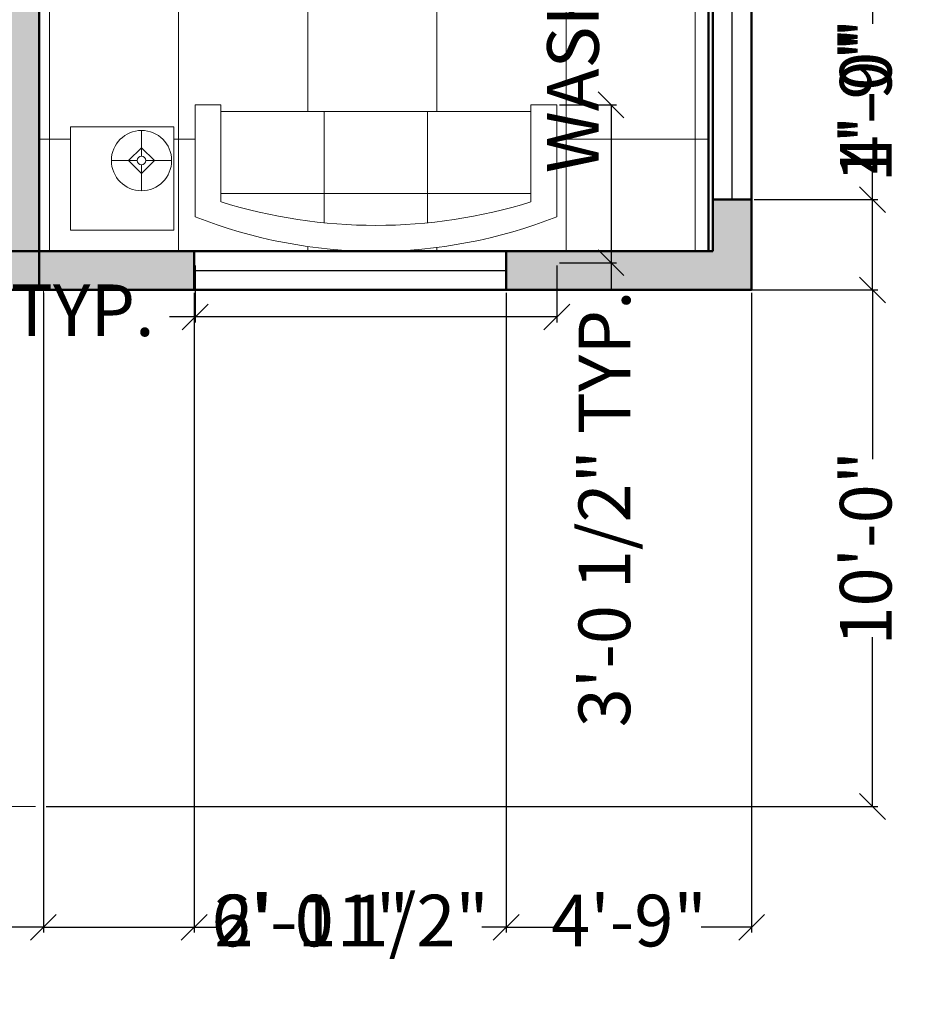
# Model space of a CAD drawing. Units: inches. Extents: x 2371 to 3019, y 129 to 700.
# Tile 10 of 14: x 2753 to 2959, y 129 to 358. Entities that reach past the tile are written whole.
import ezdxf

# ---------------------------------------------------------------- set-up
doc = ezdxf.new("R2010")
doc.units = ezdxf.units.IN
doc.linetypes.add('DASHED', pattern=[19.05, 12.7, -6.35])
for name, color, linetype, lineweight in [('A-ANNO-DIMS', 2, 'Continuous', 18), ('A-FLOR-OVHD', 20, 'DASHED', 18), ('A-FLOR-PATT', 252, 'Continuous', 13), ('A-FURN', 8, 'Continuous', 18), ('A-GLAZ', 4, 'Continuous', 25), ('A-WALL', 7, 'Continuous', 50), ('A-WALL-PATT', 8, 'Continuous', 13)]:
    doc.layers.add(name, color=color, linetype=linetype, lineweight=lineweight)
doc.styles.get("Standard").update_dxf_attribs({"font": 'arial.ttf'})
doc.dimstyles.new('ISO-25', dxfattribs={"dimtxt": 12, "dimasz": 6, "dimexe": 1.25, "dimexo": 0.625, "dimtad": 0, "dimdec": 1, "dimlunit": 3, "dimtxsty": 'Standard', "dimblk": 'OBLIQUE', "dimblk1": 'ORIGIN2', "dimblk2": 'OBLIQUE', "dimcen": 2.5, "dimadec": 0, "dimazin": 0, "dimtfac": 1, "dimtdec": 1, "dimtmove": 0, "dimatfit": 3, "dimldrblk": 'OBLIQUE', "dimfxl": 1, "dimarcsym": 0})

# ---------------------------------------------------------------- blocks, each defined once
blk = doc.blocks.new('Lamp - Table')
for p, q in [((0, 7), (0, 1)), ((0, 3), (-3, 0)), ((3, 0), (0, 3)), ((-1, 0), (-7, 0)), ((-3, 0), (0, -3)), ((0, -3), (3, 0)), ((1, 0), (7, 0)), ((0, -1), (0, -7))]:
    blk.add_line(p, q)
for radius in [7, 1]:
    blk.add_circle((0, 0), radius)
blk = doc.blocks.new('Sofa - Roundback 7 ft.')
for p, q in [((-12.00002, -32.4421), (-12.00003, -6.5971)), ((11.99997, -32.4421), (11.99998, -6.5971)), ((-36.000027, -34), (-36.000027, -11.4696)), ((-35.999844, -13.3819), (35.9998, -13.3819)), ((35.99998, -34), (35.99998, -11.4696)), ((-36.000027, -32.4421), (35.99998, -32.4421))]:
    blk.add_line(p, q)
for points in [[(-36.000027, -34), (-42.000027, -34), (-42.000027, -8)], [(41.99998, -8), (41.99998, -34), (35.99998, -34)]]:
    blk.add_lwpolyline(points)
for centre, radius, start, end in [((0, -114.25), 114.25, 68.43141, 111.5686), ((-0.00001, -127.1968), 121.1968, 72.72033, 107.2797)]:
    blk.add_arc(centre, radius, start, end)
blk = doc.blocks.new('_Oblique')
at = {"color": 0, "linetype": 'ByBlock', "lineweight": -2}
blk.add_line((-0.5, -0.5), (0.5, 0.5), dxfattribs=at)
blk = doc.blocks.new('*D20')
at = {"layer": 'A-ANNO-DIMS', "color": 0, "lineweight": -2, "transparency": 16777216}
for p, q in [((2793.86, 300.68), (2793.86, 287.46)), ((2877.86, 300.68), (2877.86, 287.46)), ((2793.86, 288.71), (2787.86, 288.71)), ((2877.86, 288.71), (2793.86, 288.71))]:
    blk.add_line(p, q, dxfattribs=at)
at = {"layer": 'Defpoints', "color": 0, "lineweight": 25, "transparency": 16777216}
for p in [(2793.86, 301.31), (2877.86, 301.31), (2793.86, 288.71)]:
    blk.add_point(p, dxfattribs=at)
at = {"layer": 'A-ANNO-DIMS', "color": 0, "lineweight": -2, "transparency": 16777216, "xscale": 6, "yscale": 6, "zscale": 6}
for p, rotation in [((2793.86, 288.71), 180.0000057391524), ((2877.86, 288.71), 5.7391524333e-06)]:
    blk.add_blockref('_Oblique', p, dxfattribs=dict(at, rotation=rotation))
at = {"layer": 'A-ANNO-DIMS', "color": 0, "transparency": 16777216, "insert": (2725.54, 288.71), "char_height": 12, "attachment_point": 5, "rotation": 0}
blk.add_mtext('SOFA 7\'-0" TYP.', dxfattribs=at)
blk = doc.blocks.new('_Origin2')
at = {"color": 0, "linetype": 'ByBlock', "lineweight": -2}
blk.add_line((-0.5, 0), (-1, 0), dxfattribs=at)
for radius in [0.5, 0.25]:
    blk.add_circle((0, 0), radius, dxfattribs=at)
blk = doc.blocks.new('*D21')
at = {"layer": 'A-ANNO-DIMS', "color": 0, "lineweight": -2, "transparency": 16777216}
for p, q in [((2878.48, 337.98), (2891.71, 337.98)), ((2890.46, 337.98), (2890.46, 301.31)), ((2878.48, 301.31), (2891.71, 301.31)), ((2890.46, 301.31), (2890.46, 295.31))]:
    blk.add_line(p, q, dxfattribs=at)
at = {"layer": 'Defpoints', "color": 0, "lineweight": 25, "transparency": 16777216}
for p in [(2877.86, 337.98), (2877.86, 301.31), (2890.46, 301.31)]:
    blk.add_point(p, dxfattribs=at)
at = {"layer": 'A-ANNO-DIMS', "color": 0, "lineweight": -2, "transparency": 16777216, "xscale": 6, "yscale": 6, "zscale": 6}
for p, rotation in [((2890.46, 337.98), 90), ((2890.46, 301.31), 270)]:
    blk.add_blockref('_Oblique', p, dxfattribs=dict(at, rotation=rotation))
at = {"layer": 'A-ANNO-DIMS', "color": 0, "transparency": 16777216, "insert": (2890.46, 244.13), "char_height": 12, "attachment_point": 5, "rotation": 90}
blk.add_mtext('3\'-0 1/2" TYP.', dxfattribs=at)
blk = doc.blocks.new('*D26')
at = {"layer": 'A-ANNO-DIMS', "color": 0, "lineweight": -2, "transparency": 16777216}
for p, q in [((2886.23, 560.02), (2881.92, 560.02)), ((2883.17, 560.02), (2883.17, 535.47)), ((2886.23, 535.47), (2881.92, 535.47)), ((2883.17, 535.47), (2883.17, 529.47))]:
    blk.add_line(p, q, dxfattribs=at)
at = {"layer": 'Defpoints', "color": 0, "lineweight": 25, "transparency": 16777216}
for p in [(2886.85, 560.02), (2883.17, 535.47), (2886.85, 535.47)]:
    blk.add_point(p, dxfattribs=at)
at = {"layer": 'A-ANNO-DIMS', "color": 0, "lineweight": -2, "transparency": 16777216, "xscale": 6, "yscale": 6, "zscale": 6}
for p, rotation in [((2883.17, 560.02), 90), ((2883.17, 535.47), 270)]:
    blk.add_blockref('_Oblique', p, dxfattribs=dict(at, rotation=rotation))
at = {"layer": 'A-ANNO-DIMS', "color": 0, "transparency": 16777216, "insert": (2883.17, 423.09), "char_height": 12, "attachment_point": 5, "rotation": 90}
blk.add_mtext('WASH BASIN 2\'-0 1/2" TYP.', dxfattribs=at)
blk = doc.blocks.new('*D53')
at = {"layer": 'A-ANNO-DIMS', "color": 0, "lineweight": -2, "transparency": 16777216}
for p, q in [((2572.61, 174.35), (2572.61, 145.68)), ((2758.61, 174.35), (2758.61, 145.68)), ((2572.61, 146.93), (2644.93, 146.93)), ((2758.61, 146.93), (2686.28, 146.93))]:
    blk.add_line(p, q, dxfattribs=at)
at = {"layer": 'Defpoints', "color": 0, "lineweight": 25, "transparency": 16777216}
for p in [(2572.61, 174.98), (2758.61, 174.98), (2758.61, 146.93)]:
    blk.add_point(p, dxfattribs=at)
at = {"layer": 'A-ANNO-DIMS', "color": 0, "lineweight": -2, "transparency": 16777216, "xscale": 6, "yscale": 6, "zscale": 6, "rotation": 180}
blk.add_blockref('_Oblique', (2572.61, 146.93), dxfattribs=at)
at = {"layer": 'A-ANNO-DIMS', "color": 0, "lineweight": -2, "transparency": 16777216, "xscale": 6, "yscale": 6, "zscale": 6}
blk.add_blockref('_Oblique', (2758.61, 146.93), dxfattribs=at)
at = {"layer": 'A-ANNO-DIMS', "color": 0, "transparency": 16777216, "insert": (2665.61, 146.93), "char_height": 12, "attachment_point": 5}
blk.add_mtext('15\'-6"', dxfattribs=at)
blk = doc.blocks.new('*D54')
at = {"layer": 'A-ANNO-DIMS', "color": 0, "lineweight": -2, "transparency": 16777216}
for p, q in [((2758.61, 294.35), (2758.61, 145.68)), ((2793.61, 294.35), (2793.61, 145.68)), ((2758.61, 146.93), (2793.61, 146.93)), ((2793.61, 146.93), (2799.61, 146.93))]:
    blk.add_line(p, q, dxfattribs=at)
at = {"layer": 'Defpoints', "color": 0, "lineweight": 25, "transparency": 16777216}
for p in [(2758.61, 294.98), (2793.61, 294.98), (2793.61, 146.93)]:
    blk.add_point(p, dxfattribs=at)
at = {"layer": 'A-ANNO-DIMS', "color": 0, "lineweight": -2, "transparency": 16777216, "xscale": 6, "yscale": 6, "zscale": 6, "rotation": 180}
blk.add_blockref('_Oblique', (2758.61, 146.93), dxfattribs=at)
at = {"layer": 'A-ANNO-DIMS', "color": 0, "lineweight": -2, "transparency": 16777216, "xscale": 6, "yscale": 6, "zscale": 6}
blk.add_blockref('_Oblique', (2793.61, 146.93), dxfattribs=at)
at = {"layer": 'A-ANNO-DIMS', "color": 0, "transparency": 16777216, "insert": (2820.94, 146.93), "char_height": 12, "attachment_point": 5}
blk.add_mtext('2\'-11"', dxfattribs=at)
blk = doc.blocks.new('*D55')
at = {"layer": 'A-ANNO-DIMS', "color": 0, "lineweight": -2, "transparency": 16777216}
for p, q in [((2793.61, 294.35), (2793.61, 145.68)), ((2866.11, 294.35), (2866.11, 145.68)), ((2793.61, 146.93), (2799.27, 146.93)), ((2866.11, 146.93), (2860.44, 146.93))]:
    blk.add_line(p, q, dxfattribs=at)
at = {"layer": 'Defpoints', "color": 0, "lineweight": 25, "transparency": 16777216}
for p in [(2793.61, 294.98), (2866.11, 294.98), (2866.11, 146.93)]:
    blk.add_point(p, dxfattribs=at)
at = {"layer": 'A-ANNO-DIMS', "color": 0, "lineweight": -2, "transparency": 16777216, "xscale": 6, "yscale": 6, "zscale": 6, "rotation": 180}
blk.add_blockref('_Oblique', (2793.61, 146.93), dxfattribs=at)
at = {"layer": 'A-ANNO-DIMS', "color": 0, "lineweight": -2, "transparency": 16777216, "xscale": 6, "yscale": 6, "zscale": 6}
blk.add_blockref('_Oblique', (2866.11, 146.93), dxfattribs=at)
at = {"layer": 'A-ANNO-DIMS', "color": 0, "transparency": 16777216, "insert": (2829.86, 146.93), "char_height": 12, "attachment_point": 5}
blk.add_mtext('6\'-0 1/2"', dxfattribs=at)
blk = doc.blocks.new('*D56')
at = {"layer": 'A-ANNO-DIMS', "color": 0, "lineweight": -2, "transparency": 16777216}
for p, q in [((2866.11, 294.35), (2866.11, 145.68)), ((2923.11, 294.35), (2923.11, 145.68)), ((2866.11, 146.93), (2877.79, 146.93)), ((2923.11, 146.93), (2911.42, 146.93))]:
    blk.add_line(p, q, dxfattribs=at)
at = {"layer": 'Defpoints', "color": 0, "lineweight": 25, "transparency": 16777216}
for p in [(2866.11, 294.98), (2923.11, 294.98), (2923.11, 146.93)]:
    blk.add_point(p, dxfattribs=at)
at = {"layer": 'A-ANNO-DIMS', "color": 0, "lineweight": -2, "transparency": 16777216, "xscale": 6, "yscale": 6, "zscale": 6, "rotation": 180}
blk.add_blockref('_Oblique', (2866.11, 146.93), dxfattribs=at)
at = {"layer": 'A-ANNO-DIMS', "color": 0, "lineweight": -2, "transparency": 16777216, "xscale": 6, "yscale": 6, "zscale": 6}
blk.add_blockref('_Oblique', (2923.11, 146.93), dxfattribs=at)
at = {"layer": 'A-ANNO-DIMS', "color": 0, "transparency": 16777216, "insert": (2894.61, 146.93), "char_height": 12, "attachment_point": 5}
blk.add_mtext('4\'-9"', dxfattribs=at)
blk = doc.blocks.new('*D57')
at = {"layer": 'A-ANNO-DIMS', "color": 0, "lineweight": -2, "transparency": 16777216}
for p, q in [((2759.23, 294.98), (2952.41, 294.98)), ((2951.16, 294.98), (2951.16, 255.65)), ((2951.16, 174.98), (2951.16, 214.3)), ((2759.23, 174.98), (2952.41, 174.98))]:
    blk.add_line(p, q, dxfattribs=at)
at = {"layer": 'Defpoints', "color": 0, "lineweight": 25, "transparency": 16777216}
for p in [(2758.61, 294.98), (2758.61, 174.98), (2951.16, 174.98)]:
    blk.add_point(p, dxfattribs=at)
at = {"layer": 'A-ANNO-DIMS', "color": 0, "lineweight": -2, "transparency": 16777216, "xscale": 6, "yscale": 6, "zscale": 6}
for p, rotation in [((2951.16, 294.98), 90), ((2951.16, 174.98), 270)]:
    blk.add_blockref('_Oblique', p, dxfattribs=dict(at, rotation=rotation))
at = {"layer": 'A-ANNO-DIMS', "color": 0, "transparency": 16777216, "insert": (2951.16, 234.98), "char_height": 12, "attachment_point": 5, "rotation": 90}
blk.add_mtext('10\'-0"', dxfattribs=at)
blk = doc.blocks.new('*D61')
at = {"layer": 'A-ANNO-DIMS', "color": 0, "lineweight": -2, "transparency": 16777216}
for p, q in [((2951.16, 315.98), (2951.16, 321.98)), ((2923.73, 315.98), (2952.41, 315.98)), ((2951.16, 294.98), (2951.16, 315.98)), ((2923.73, 294.98), (2952.41, 294.98))]:
    blk.add_line(p, q, dxfattribs=at)
at = {"layer": 'Defpoints', "color": 0, "lineweight": 25, "transparency": 16777216}
for p in [(2923.11, 315.98), (2951.16, 315.98), (2923.11, 294.98)]:
    blk.add_point(p, dxfattribs=at)
at = {"layer": 'A-ANNO-DIMS', "color": 0, "lineweight": -2, "transparency": 16777216, "xscale": 6, "yscale": 6, "zscale": 6}
for p, rotation in [((2951.16, 315.98), 90), ((2951.16, 294.98), 270)]:
    blk.add_blockref('_Oblique', p, dxfattribs=dict(at, rotation=rotation))
at = {"layer": 'A-ANNO-DIMS', "color": 0, "transparency": 16777216, "insert": (2951.16, 337.99), "char_height": 12, "attachment_point": 5, "rotation": 90}
blk.add_mtext('1\'-9"', dxfattribs=at)
blk = doc.blocks.new('*D62')
at = {"layer": 'A-ANNO-DIMS', "color": 0, "lineweight": -2, "transparency": 16777216}
for p, q in [((2923.73, 363.98), (2952.41, 363.98)), ((2951.16, 363.98), (2951.16, 356.79)), ((2951.16, 315.98), (2951.16, 323.16)), ((2923.73, 315.98), (2952.41, 315.98))]:
    blk.add_line(p, q, dxfattribs=at)
at = {"layer": 'Defpoints', "color": 0, "lineweight": 25, "transparency": 16777216}
for p in [(2923.11, 363.98), (2951.16, 363.98), (2923.11, 315.98)]:
    blk.add_point(p, dxfattribs=at)
at = {"layer": 'A-ANNO-DIMS', "color": 0, "lineweight": -2, "transparency": 16777216, "xscale": 6, "yscale": 6, "zscale": 6}
for p, rotation in [((2951.16, 363.98), 90), ((2951.16, 315.98), 270)]:
    blk.add_blockref('_Oblique', p, dxfattribs=dict(at, rotation=rotation))
at = {"layer": 'A-ANNO-DIMS', "color": 0, "transparency": 16777216, "insert": (2951.16, 339.98), "char_height": 12, "attachment_point": 5, "rotation": 90}
blk.add_mtext('4\'-0"', dxfattribs=at)

msp = doc.modelspace()

# ---------------------------------------------------------------- hatches: boundary and pattern name
at = {"layer": 'A-FLOR-PATT'}
h = msp.add_hatch(dxfattribs=at)
h.set_pattern_fill('_USER', color=256, scale=30, pattern_type=0)
h.set_pattern_definition([(0, (0, 0), (0, 30), [])])
h.paths.add_polyline_path([(2913.11, 498.98), (2827.61, 498.98), (2827.61, 531.98), (2832.11, 531.98), (2832.11, 537.98), (2833.61, 537.98), (2833.61, 605.98), (2818.35, 605.98, -1), (2796.86, 605.98), (2781.61, 605.98), (2781.61, 603.98), (2781.61, 533.98), (2757.61, 533.98), (2757.61, 531.98), (2797.61, 531.98), (2797.61, 522.98), (2757.61, 522.98), (2757.61, 516.98), (2754.59, 516.98), (2772.52, 485.76), (2771.01, 484.89), (2770.98, 484.93, -0.097552), (2757.61, 481.1), (2757.61, 422.48), (2837.61, 422.48), (2837.61, 362.48), (2757.61, 362.48), (2757.61, 303.98), (2835.86, 303.98, -0.09439), (2793.86, 311.98), (2793.86, 337.98), (2799.86, 337.98), (2799.86, 336.42), (2871.86, 336.42), (2871.86, 337.98), (2877.86, 337.98), (2877.86, 311.98, -0.09439), (2835.86, 303.98), (2913.11, 303.98), (2913.11, 383.18), (2904.11, 383.18), (2904.11, 419.18), (2913.11, 419.18)])
h.paths.add_polyline_path([(2788.88, 332.88), (2788.88, 308.88), (2764.88, 308.88), (2764.88, 332.88)], flags=16)
h.paths.add_polyline_path([(2788.4, 325.04, -1), (2774.4, 325.04, -1)], flags=0)
h.paths.add_polyline_path([(2781.4, 328.04), (2784.4, 325.04), (2781.4, 322.04), (2778.4, 325.04)], flags=0)
h.paths.add_polyline_path([(2782.4, 325.04, -1), (2780.4, 325.04, -1)], flags=0)
h.paths.add_polyline_path([(2748.61, 480.99), (2754.51, 480.98, 0.119303), (2770.98, 484.93), (2753.07, 516.1), (2754.59, 516.98), (2748.61, 516.98), (2748.61, 539.98), (2712.61, 539.98), (2665.11, 539.98, -0.09439), (2707.11, 531.98), (2707.11, 505.98), (2701.11, 505.98), (2701.11, 507.53), (2629.11, 507.53), (2629.11, 505.98), (2623.11, 505.98), (2623.11, 531.98, -0.09439), (2665.11, 539.98), (2581.61, 539.98), (2581.61, 522.98), (2581.61, 477.98, -0.131044), (2589.61, 507.98), (2615.61, 507.98), (2615.61, 501.98), (2614.05, 501.98), (2614.05, 453.98), (2615.61, 453.98), (2615.61, 447.98), (2589.61, 447.98, -0.131044), (2581.61, 477.98), (2581.61, 432.98), (2572.61, 432.98, 0.119303), (2556.14, 428.99), (2574.12, 397.85), (2572.61, 396.98), (2578.61, 396.98), (2581.61, 396.98), (2581.61, 390.98), (2748.61, 390.98)])
h.paths.add_polyline_path([(2683.1, 447.25), (2652.43, 447.25), (2652.43, 492.22), (2683.1, 492.22)], flags=16)
h.paths.add_polyline_path([(2682.1, 448.25), (2653.43, 448.25), (2653.43, 491.22), (2682.1, 491.22)], flags=0)
h.paths.add_polyline_path([(2613.58, 512.06), (2589.58, 512.06), (2589.58, 536.06), (2613.58, 536.06)], flags=16)
h.paths.add_polyline_path([(2599.1, 528.22, -1), (2613.1, 528.22, -1)], flags=0)
h.paths.add_polyline_path([(2609.1, 528.22), (2606.1, 525.22), (2603.1, 528.22), (2606.1, 531.22)], flags=0)
h.paths.add_polyline_path([(2607.1, 528.22, -1), (2605.1, 528.22, -1)], flags=0)
h.paths.add_polyline_path([(2581.61, 522.98), (2581.61, 621.98), (2572.61, 621.98), (2572.61, 522.98), (2572.61, 500.98), (2565.85, 500.98), (2565.85, 500.15), (2564.82, 500.15), (2561.16, 500.19), (2561.16, 500.17), (2560.13, 500.3), (2560.22, 500.98), (2556.38, 500.98), (2556.43, 500.22), (2555.4, 500.14), (2555.34, 500.98), (2551.07, 500.98), (2551.07, 500.15), (2550.04, 500.15), (2547.64, 500.19), (2547.64, 500.15), (2546.61, 500.15), (2541.79, 500.22), (2540.72, 500.13), (2540.65, 500.98), (2533.37, 500.98), (2533.37, 500.15), (2532.34, 500.15), (2529.13, 500.21), (2529.12, 500.13), (2528.09, 500.22), (2528.16, 500.98), (2523.23, 500.98), (2523.23, 500.15), (2522.2, 500.15), (2519.8, 500.21), (2519.8, 500.15), (2518.77, 500.15), (2514.45, 500.26), (2514.44, 500.14), (2513.41, 500.22), (2513.47, 500.98), (2509.62, 500.98), (2509.71, 500.3), (2508.69, 500.17), (2508.58, 500.98), (2505.03, 500.98), (2505.03, 500.15), (2503.99, 500.15), (2501.07, 500.29), (2501.07, 500.15), (2500.04, 500.15), (2496.44, 500.37), (2496.44, 500.15), (2495.4, 500.15), (2492.55, 500.41), (2492.18, 500.35), (2492.09, 500.98), (2486.11, 500.98), (2486.11, 524.98), (2486.11, 531.98), (2490.61, 531.98), (2490.61, 537.98), (2492.11, 537.98), (2492.11, 605.98), (2476.85, 605.98, -1), (2455.36, 605.98), (2440.11, 605.98), (2440.11, 533.98), (2416.11, 533.98), (2416.11, 605.98), (2416.11, 621.98), (2536.61, 621.98), (2536.61, 630.98), (2407.11, 630.98), (2407.11, 363.98), (2416.11, 363.98), (2416.11, 431.48), (2496.11, 431.48), (2496.11, 371.48), (2416.11, 371.48), (2416.11, 303.98), (2494.36, 303.98, -0.09439), (2452.36, 311.98), (2452.36, 337.98), (2458.36, 337.98), (2458.36, 336.42), (2530.36, 336.42), (2530.36, 337.98), (2536.36, 337.98), (2536.36, 311.98, -0.09439), (2494.36, 303.98), (2572.61, 303.98), (2572.61, 381.98), (2572.61, 396.98), (2554.61, 428.15), (2556.12, 429.03), (2556.14, 428.99, -0.119303), (2572.61, 432.98), (2578.61, 432.98), (2581.61, 432.98)])
h.paths.add_polyline_path([(2450.11, 500.98), (2444.5, 500.98), (2444.44, 500.14), (2443.41, 500.22), (2443.47, 500.98), (2439.62, 500.98), (2439.71, 500.3), (2438.69, 500.17), (2438.58, 500.98), (2435.02, 500.98), (2435.02, 500.15), (2433.99, 500.15), (2433.99, 500.98), (2431.07, 500.98), (2431.07, 500.15), (2430.04, 500.15), (2430.04, 500.98), (2426.43, 500.98), (2426.43, 500.15), (2425.4, 500.15), (2425.4, 500.98), (2423.13, 500.98), (2423.2, 500.5), (2422.18, 500.35), (2422.09, 500.98), (2416.11, 500.98), (2416.11, 524.98), (2416.11, 531.98), (2450.11, 531.98), (2450.11, 522.98)], flags=16)
h.paths.add_polyline_path([(2449.11, 501.98), (2417.11, 501.98), (2417.11, 522.98), (2417.11, 523.98), (2449.11, 523.98)], flags=0)
h.paths.add_polyline_path([(2420.7, 510.73), (2419.36, 520.07), (2420.38, 520.22), (2421.74, 510.73), (2425.4, 510.73), (2425.4, 520.07), (2426.43, 520.07), (2426.43, 510.73), (2430.04, 510.73), (2430.04, 520.07), (2431.07, 520.07), (2431.07, 510.73), (2433.99, 510.73), (2433.99, 520.07), (2435.02, 520.07), (2435.02, 510.73), (2437.35, 510.73), (2436.18, 519.93), (2437.2, 520.06), (2438.39, 510.73), (2444.17, 510.73), (2444.85, 520.08), (2445.88, 520.01), (2445.21, 510.73)], flags=0)
h.paths.add_polyline_path([(2446.94, 336.11), (2446.94, 312.11), (2422.94, 312.11), (2422.94, 336.11)], flags=16)
h.paths.add_polyline_path([(2446.46, 328.27, -1), (2432.46, 328.27, -1)], flags=0)
h.paths.add_polyline_path([(2439.46, 331.27), (2442.46, 328.27), (2439.46, 325.27), (2436.46, 328.27)], flags=0)
h.paths.add_polyline_path([(2440.46, 328.27, -1), (2438.46, 328.27, -1)], flags=0)
h.paths.add_polyline_path([(2816, 444.88), (2866.87, 444.88), (2866.87, 463.54), (2816, 463.54)], flags=24)
h.paths.add_polyline_path([(2794.21, 558.3), (2833.34, 558.3), (2833.34, 576.96), (2794.21, 576.96)], flags=24)
h.paths.add_polyline_path([(2651.69, 411.53), (2711.04, 411.53), (2711.04, 430.19), (2651.69, 430.19)], flags=24)
h.paths.add_polyline_path([(2494.09, 444.88), (2544.97, 444.88), (2544.97, 463.54), (2494.09, 463.54)], flags=24)
h.paths.add_polyline_path([(2444.55, 565.02), (2483.69, 565.02), (2483.69, 583.68), (2444.55, 583.68)], flags=24)
h = msp.add_hatch(dxfattribs=at)
h.set_pattern_fill('_USER', color=256, scale=30, angle=90, pattern_type=0)
h.set_pattern_definition([(90, (0, 0), (-30, 2e-15), [])])
h.paths.add_polyline_path([(2913.11, 498.98), (2827.61, 498.98), (2827.61, 531.98), (2832.11, 531.98), (2832.11, 537.98), (2833.61, 537.98), (2833.61, 605.98), (2818.35, 605.98, -1), (2796.86, 605.98), (2781.61, 605.98), (2781.61, 603.98), (2781.61, 533.98), (2757.61, 533.98), (2757.61, 531.98), (2797.61, 531.98), (2797.61, 522.98), (2757.61, 522.98), (2757.61, 516.98), (2754.59, 516.98), (2772.52, 485.76), (2771.01, 484.89), (2770.98, 484.93, -0.097552), (2757.61, 481.1), (2757.61, 422.48), (2837.61, 422.48), (2837.61, 362.48), (2757.61, 362.48), (2757.61, 303.98), (2835.86, 303.98, -0.09439), (2793.86, 311.98), (2793.86, 337.98), (2799.86, 337.98), (2799.86, 336.42), (2871.86, 336.42), (2871.86, 337.98), (2877.86, 337.98), (2877.86, 311.98, -0.09439), (2835.86, 303.98), (2913.11, 303.98), (2913.11, 383.18), (2904.11, 383.18), (2904.11, 419.18), (2913.11, 419.18)])
h.paths.add_polyline_path([(2788.88, 332.88), (2788.88, 308.88), (2764.88, 308.88), (2764.88, 332.88)], flags=16)
h.paths.add_polyline_path([(2788.4, 325.04, -1), (2774.4, 325.04, -1)], flags=0)
h.paths.add_polyline_path([(2781.4, 328.04), (2784.4, 325.04), (2781.4, 322.04), (2778.4, 325.04)], flags=0)
h.paths.add_polyline_path([(2782.4, 325.04, -1), (2780.4, 325.04, -1)], flags=0)
h.paths.add_polyline_path([(2748.61, 480.99), (2754.51, 480.98, 0.119303), (2770.98, 484.93), (2753.07, 516.1), (2754.59, 516.98), (2748.61, 516.98), (2748.61, 539.98), (2712.61, 539.98), (2665.11, 539.98, -0.09439), (2707.11, 531.98), (2707.11, 505.98), (2701.11, 505.98), (2701.11, 507.53), (2629.11, 507.53), (2629.11, 505.98), (2623.11, 505.98), (2623.11, 531.98, -0.09439), (2665.11, 539.98), (2581.61, 539.98), (2581.61, 522.98), (2581.61, 477.98, -0.131044), (2589.61, 507.98), (2615.61, 507.98), (2615.61, 501.98), (2614.05, 501.98), (2614.05, 453.98), (2615.61, 453.98), (2615.61, 447.98), (2589.61, 447.98, -0.131044), (2581.61, 477.98), (2581.61, 432.98), (2572.61, 432.98, 0.119303), (2556.14, 428.99), (2574.12, 397.85), (2572.61, 396.98), (2578.61, 396.98), (2581.61, 396.98), (2581.61, 390.98), (2748.61, 390.98)])
h.paths.add_polyline_path([(2683.1, 447.25), (2652.43, 447.25), (2652.43, 492.22), (2683.1, 492.22)], flags=16)
h.paths.add_polyline_path([(2682.1, 448.25), (2653.43, 448.25), (2653.43, 491.22), (2682.1, 491.22)], flags=0)
h.paths.add_polyline_path([(2613.58, 512.06), (2589.58, 512.06), (2589.58, 536.06), (2613.58, 536.06)], flags=16)
h.paths.add_polyline_path([(2599.1, 528.22, -1), (2613.1, 528.22, -1)], flags=0)
h.paths.add_polyline_path([(2609.1, 528.22), (2606.1, 525.22), (2603.1, 528.22), (2606.1, 531.22)], flags=0)
h.paths.add_polyline_path([(2607.1, 528.22, -1), (2605.1, 528.22, -1)], flags=0)
h.paths.add_polyline_path([(2581.61, 522.98), (2581.61, 621.98), (2572.61, 621.98), (2572.61, 522.98), (2572.61, 500.98), (2565.85, 500.98), (2565.85, 500.15), (2564.82, 500.15), (2561.16, 500.19), (2561.16, 500.17), (2560.13, 500.3), (2560.22, 500.98), (2556.38, 500.98), (2556.43, 500.22), (2555.4, 500.14), (2555.34, 500.98), (2551.07, 500.98), (2551.07, 500.15), (2550.04, 500.15), (2547.64, 500.19), (2547.64, 500.15), (2546.61, 500.15), (2541.79, 500.22), (2540.72, 500.13), (2540.65, 500.98), (2533.37, 500.98), (2533.37, 500.15), (2532.34, 500.15), (2529.13, 500.21), (2529.12, 500.13), (2528.09, 500.22), (2528.16, 500.98), (2523.23, 500.98), (2523.23, 500.15), (2522.2, 500.15), (2519.8, 500.21), (2519.8, 500.15), (2518.77, 500.15), (2514.45, 500.26), (2514.44, 500.14), (2513.41, 500.22), (2513.47, 500.98), (2509.62, 500.98), (2509.71, 500.3), (2508.69, 500.17), (2508.58, 500.98), (2505.03, 500.98), (2505.03, 500.15), (2503.99, 500.15), (2501.07, 500.29), (2501.07, 500.15), (2500.04, 500.15), (2496.44, 500.37), (2496.44, 500.15), (2495.4, 500.15), (2492.55, 500.41), (2492.18, 500.35), (2492.09, 500.98), (2486.11, 500.98), (2486.11, 524.98), (2486.11, 531.98), (2490.61, 531.98), (2490.61, 537.98), (2492.11, 537.98), (2492.11, 605.98), (2476.85, 605.98, -1), (2455.36, 605.98), (2440.11, 605.98), (2440.11, 533.98), (2416.11, 533.98), (2416.11, 605.98), (2416.11, 621.98), (2536.61, 621.98), (2536.61, 630.98), (2407.11, 630.98), (2407.11, 363.98), (2416.11, 363.98), (2416.11, 431.48), (2496.11, 431.48), (2496.11, 371.48), (2416.11, 371.48), (2416.11, 303.98), (2494.36, 303.98, -0.09439), (2452.36, 311.98), (2452.36, 337.98), (2458.36, 337.98), (2458.36, 336.42), (2530.36, 336.42), (2530.36, 337.98), (2536.36, 337.98), (2536.36, 311.98, -0.09439), (2494.36, 303.98), (2572.61, 303.98), (2572.61, 381.98), (2572.61, 396.98), (2554.61, 428.15), (2556.12, 429.03), (2556.14, 428.99, -0.119303), (2572.61, 432.98), (2578.61, 432.98), (2581.61, 432.98)])
h.paths.add_polyline_path([(2450.11, 500.98), (2444.5, 500.98), (2444.44, 500.14), (2443.41, 500.22), (2443.47, 500.98), (2439.62, 500.98), (2439.71, 500.3), (2438.69, 500.17), (2438.58, 500.98), (2435.02, 500.98), (2435.02, 500.15), (2433.99, 500.15), (2433.99, 500.98), (2431.07, 500.98), (2431.07, 500.15), (2430.04, 500.15), (2430.04, 500.98), (2426.43, 500.98), (2426.43, 500.15), (2425.4, 500.15), (2425.4, 500.98), (2423.13, 500.98), (2423.2, 500.5), (2422.18, 500.35), (2422.09, 500.98), (2416.11, 500.98), (2416.11, 524.98), (2416.11, 531.98), (2450.11, 531.98), (2450.11, 522.98)], flags=16)
h.paths.add_polyline_path([(2449.11, 501.98), (2417.11, 501.98), (2417.11, 522.98), (2417.11, 523.98), (2449.11, 523.98)], flags=0)
h.paths.add_polyline_path([(2420.7, 510.73), (2419.36, 520.07), (2420.38, 520.22), (2421.74, 510.73), (2425.4, 510.73), (2425.4, 520.07), (2426.43, 520.07), (2426.43, 510.73), (2430.04, 510.73), (2430.04, 520.07), (2431.07, 520.07), (2431.07, 510.73), (2433.99, 510.73), (2433.99, 520.07), (2435.02, 520.07), (2435.02, 510.73), (2437.35, 510.73), (2436.18, 519.93), (2437.2, 520.06), (2438.39, 510.73), (2444.17, 510.73), (2444.85, 520.08), (2445.88, 520.01), (2445.21, 510.73)], flags=0)
h.paths.add_polyline_path([(2446.94, 336.11), (2446.94, 312.11), (2422.94, 312.11), (2422.94, 336.11)], flags=16)
h.paths.add_polyline_path([(2446.46, 328.27, -1), (2432.46, 328.27, -1)], flags=0)
h.paths.add_polyline_path([(2439.46, 331.27), (2442.46, 328.27), (2439.46, 325.27), (2436.46, 328.27)], flags=0)
h.paths.add_polyline_path([(2440.46, 328.27, -1), (2438.46, 328.27, -1)], flags=0)
h.paths.add_polyline_path([(2816, 444.88), (2866.87, 444.88), (2866.87, 463.54), (2816, 463.54)], flags=24)
h.paths.add_polyline_path([(2794.21, 558.3), (2833.34, 558.3), (2833.34, 576.96), (2794.21, 576.96)], flags=24)
h.paths.add_polyline_path([(2651.69, 411.53), (2711.04, 411.53), (2711.04, 430.19), (2651.69, 430.19)], flags=24)
h.paths.add_polyline_path([(2494.09, 444.88), (2544.97, 444.88), (2544.97, 463.54), (2494.09, 463.54)], flags=24)
h.paths.add_polyline_path([(2444.55, 565.02), (2483.69, 565.02), (2483.69, 583.68), (2444.55, 583.68)], flags=24)
at = {"layer": 'A-WALL-PATT'}
h = msp.add_hatch(color=256, dxfattribs=at)
h.dxf.hatch_style = 1
h.paths.add_polyline_path([(2536.61, 630.98), (2407.11, 630.98), (2407.11, 363.98), (2416.11, 363.98), (2416.11, 498.98), (2416.11, 522.98), (2416.11, 531.98), (2416.11, 603.98), (2416.11, 621.98), (2536.61, 621.98)])
h.paths.add_polyline_path([(2630.98, 630.98), (2560.61, 630.98), (2560.61, 621.98), (2630.98, 621.98)])
h.paths.add_polyline_path([(2878.11, 630.98), (2699.23, 630.98), (2699.23, 621.98), (2878.11, 621.98)])
h.paths.add_polyline_path([(2496.61, 621.98), (2492.11, 621.98), (2492.11, 569.98), (2496.61, 569.98)], flags=17)
h.paths.add_polyline_path([(2581.61, 621.98), (2572.61, 621.98), (2572.61, 522.98), (2572.61, 498.98), (2572.61, 432.98), (2578.61, 432.98), (2581.61, 432.98), (2581.61, 522.98)])
h.paths.add_polyline_path([(2572.61, 531.98), (2486.11, 531.98), (2486.11, 522.98), (2572.61, 522.98)])
h.paths.add_polyline_path([(2450.11, 531.98), (2440.11, 531.98), (2416.11, 531.98), (2416.11, 522.98), (2450.11, 522.98)], flags=17)
h.paths.add_polyline_path([(2416.11, 315.98), (2407.11, 315.98), (2407.11, 294.98), (2458.11, 294.98), (2458.11, 303.98), (2416.11, 303.98)])
h.paths.add_polyline_path([(2757.61, 303.98), (2530.61, 303.98), (2530.61, 294.98), (2757.61, 294.98)])
h.paths.add_polyline_path([(2581.61, 381.98), (2605.61, 381.98), (2617.61, 381.98), (2617.61, 390.98), (2581.61, 390.98), (2581.61, 396.98), (2572.61, 396.98), (2572.61, 381.98), (2572.61, 303.98), (2581.61, 303.98)])
h.paths.add_polyline_path([(2757.61, 480.98), (2748.61, 480.98), (2748.61, 381.98), (2748.61, 303.98), (2757.61, 303.98), (2757.61, 381.98), (2757.61, 422.48)])
h.paths.add_polyline_path([(2797.61, 531.98), (2757.61, 531.98), (2757.61, 603.98), (2757.61, 621.98), (2748.61, 621.98), (2748.61, 516.99), (2754.59, 516.98), (2757.61, 516.98), (2757.61, 522.98), (2797.61, 522.98)])
h.paths.add_polyline_path([(2913.11, 531.98), (2827.61, 531.98), (2827.61, 522.98), (2913.11, 522.98)])
h.paths.add_polyline_path([(2923.11, 630.98), (2902.11, 630.98), (2902.11, 621.98), (2914.11, 621.98), (2914.11, 363.98), (2923.11, 363.98)])
h.paths.add_polyline_path([(2923.11, 315.98), (2914.11, 315.98), (2914.11, 303.98), (2866.11, 303.98), (2866.11, 294.98), (2923.11, 294.98)])
h.paths.add_polyline_path([(2793.61, 303.98), (2757.61, 303.98), (2757.61, 294.98), (2793.61, 294.98)])

# ---------------------------------------------------------------- linework, layer by layer
at = {"layer": 'A-FLOR-OVHD'}
msp.add_lwpolyline([(2572.61, 294.98), (2572.61, 174.98), (2758.61, 174.98), (2758.61, 294.98)], dxfattribs=at)
at = {"layer": 'A-FURN'}
msp.add_lwpolyline([(2764.88, 308.88), (2788.88, 308.88), (2788.88, 332.88), (2764.88, 332.88)], close=True, dxfattribs=at)
at = {"layer": 'A-GLAZ'}
for p, q in [((2918.61, 315.98), (2918.61, 363.98)), ((2793.61, 299.48), (2866.11, 299.48))]:
    msp.add_line(p, q, dxfattribs=at)
at = {"layer": 'A-WALL'}
for p, q in [((2923.11, 294.98), (2923.11, 630.98)), ((2914.11, 303.98), (2914.11, 621.98)), ((2913.11, 303.98), (2913.11, 498.98)), ((2757.61, 303.98), (2757.61, 381.98)), ((2914.11, 315.98), (2923.11, 315.98)), ((2416.11, 303.98), (2914.11, 303.98)), ((2757.61, 294.98), (2757.61, 303.98)), ((2793.61, 294.98), (2793.61, 303.98)), ((2793.61, 303.98), (2793.61, 294.98)), ((2866.11, 303.98), (2866.11, 294.98)), ((2407.11, 294.98), (2923.11, 294.98))]:
    msp.add_line(p, q, dxfattribs=at)

# ---------------------------------------------------------------- block references
at = {"layer": 'A-FURN', "rotation": 180.0000057391524}
msp.add_blockref('Sofa - Roundback 7 ft.', (2835.86, 303.98), dxfattribs=at)
at = {"layer": 'A-FURN'}
msp.add_blockref('Lamp - Table', (2781.4, 325.04), dxfattribs=at)

# ---------------------------------------------------------------- dimensions: what is measured, and where the dimension line sits
at = {"layer": 'A-ANNO-DIMS'}
for base, p1, p2, angle, text, picture, middle in [((2883.1676, 535.4732), (2886.8502, 560.0241), (2886.8502, 535.4732), 270, 'WASH BASIN <> TYP.', '*D26', (2883.1676, 423.0911)), ((2890.46, 301.31), (2877.86, 337.98), (2877.86, 301.31), 270, '<> TYP.', '*D21', (2890.46, 244.13)), ((2793.86, 288.71), (2877.86, 301.31), (2793.86, 301.31), 180, 'SOFA <> TYP.', '*D20', (2725.54, 288.71))]:
    dim = msp.add_linear_dim(base=base, p1=p1, p2=p2, angle=angle, text=text, dimstyle='ISO-25', override={"dimdec": 1, "dimrnd": 0, "dimzin": 1, "dimlunit": 4, "dimfrac": 2}, dxfattribs=at)
    dim.commit()
    dim.dimension.update_dxf_attribs({"geometry": picture, "text_midpoint": middle})
for base, p1, p2, picture, middle in [((2951.16, 363.98), (2923.11, 315.98), (2923.11, 363.98), '*D62', (2951.16, 339.98)), ((2951.16, 315.98), (2923.11, 294.98), (2923.11, 315.98), '*D61', (2951.16, 337.99)), ((2951.16, 174.98), (2758.61, 294.98), (2758.61, 174.98), '*D57', (2951.16, 234.98))]:
    dim = msp.add_linear_dim(base=base, p1=p1, p2=p2, angle=90, dimstyle='ISO-25', override={"dimdec": 1, "dimlfac": 1, "dimrnd": 0, "dimzin": 1, "dimdsep": 46, "dimlunit": 4, "dimfrac": 2}, dxfattribs=at)
    dim.commit()
    dim.dimension.update_dxf_attribs({"geometry": picture, "text_midpoint": middle})
for base, p1, p2, picture, middle in [((2793.61, 146.93), (2758.61, 294.98), (2793.61, 294.98), '*D54', (2820.94, 146.93)), ((2866.11, 146.93), (2793.61, 294.98), (2866.11, 294.98), '*D55', (2829.86, 146.93)), ((2923.11, 146.93), (2866.11, 294.98), (2923.11, 294.98), '*D56', (2894.61, 146.93)), ((2758.61, 146.93), (2572.61, 174.98), (2758.61, 174.98), '*D53', (2665.61, 146.93))]:
    dim = msp.add_linear_dim(base=base, p1=p1, p2=p2, dimstyle='ISO-25', override={"dimdec": 1, "dimlfac": 1, "dimrnd": 0, "dimzin": 1, "dimdsep": 46, "dimlunit": 4, "dimfrac": 2}, dxfattribs=at)
    dim.commit()
    dim.dimension.update_dxf_attribs({"geometry": picture, "text_midpoint": middle})

doc.saveas('drawing.dxf')
